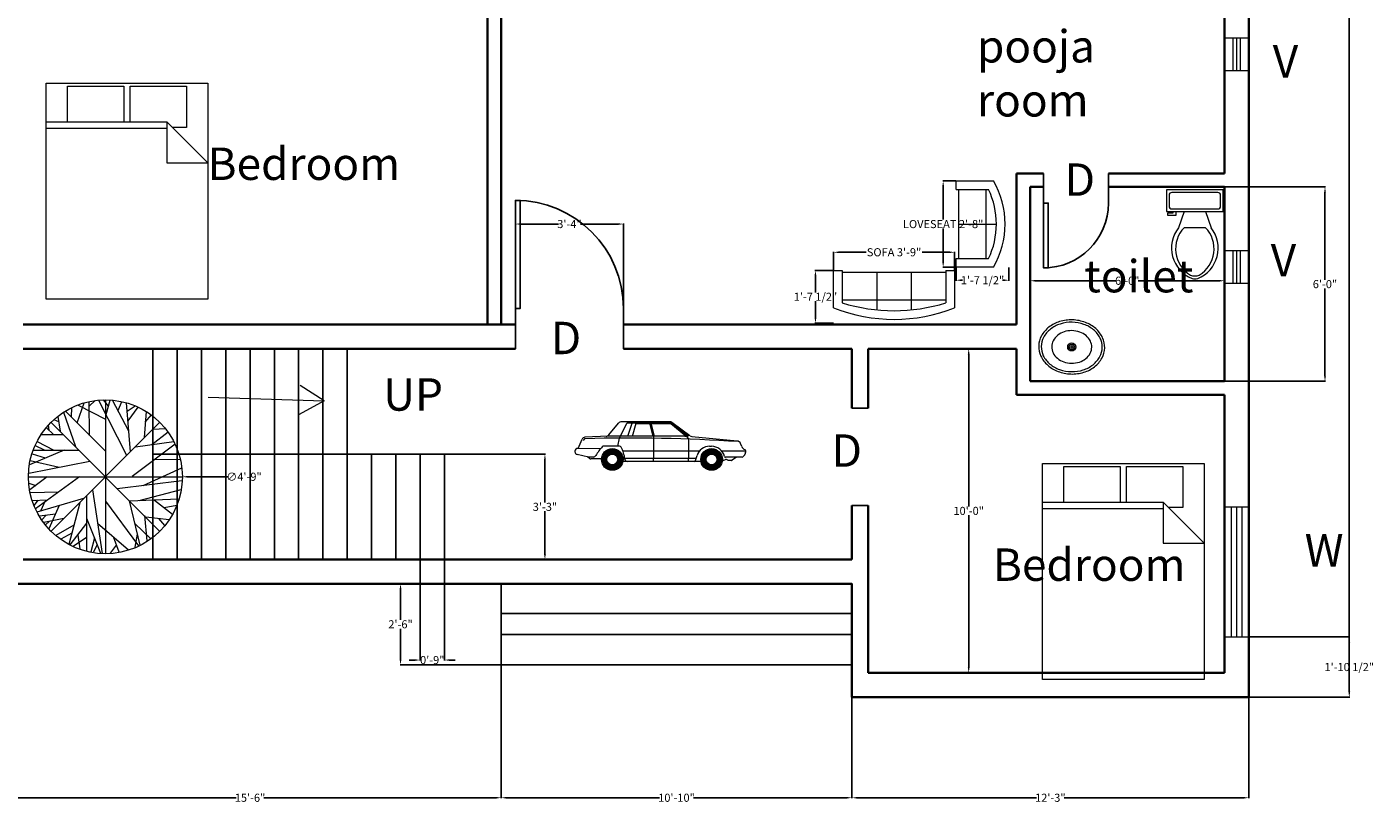
# Model space of a CAD drawing. Units: inches. Extents: x 751 to 1500, y 610 to 1297.
# Tile 2 of 4: x 1001 to 1500, y 610 to 898. Entities that reach past the tile are written whole.
import ezdxf

# ---------------------------------------------------------------- set-up
doc = ezdxf.new("R2010")
doc.units = ezdxf.units.IN
doc.header["$MEASUREMENT"] = 0
doc.layers.get('0').update_dxf_attribs({"color": 1})
for name, color, linetype, lineweight in [('A-ANNO-DIMS', 5, 'Continuous', 18), ('A-ANNO-SYMB', 7, 'Continuous', 18), ('A-ANNO-TEXT', 7, 'Continuous', 18), ('A-AREA-IDEN', 7, 'Continuous', 25), ('A-FLOR-FIXT', 9, 'Continuous', 18), ('A-FURN', 8, 'Continuous', 18), ('A-SITE-VEHI', 8, 'Continuous', 13), ('door', 2, 'Continuous', 25), ('L-PLNT', 3, 'Continuous', 13), ('stair', 130, 'Continuous', 25), ('wall', 6, 'Continuous', 35), ('windows', 70, 'Continuous', 18)]:
    doc.layers.add(name, color=color, linetype=linetype, lineweight=lineweight)
doc.styles.get("Standard").update_dxf_attribs({"font": 'arial.ttf'})
doc.dimstyles.get("Standard").update_dxf_attribs({"dimtxt": 3, "dimasz": 2, "dimexe": 0.18, "dimexo": 0.0625, "dimgap": 0.09, "dimtad": 0, "dimtih": 1, "dimtoh": 1, "dimdec": 0, "dimzin": 0, "dimdsep": 46, "dimlunit": 3, "dimtxsty": 'Standard', "dimcen": 0.09, "dimadec": 0, "dimazin": 0, "dimtfac": 1, "dimtdec": 0, "dimtofl": 0, "dimtmove": 0, "dimatfit": 3, "dimfxl": 1, "dimtolj": 1, "dimtzin": 0, "dimarcsym": 0})

# ---------------------------------------------------------------- blocks, each defined once
blk = doc.blocks.new('*U5')
for p, q in [((-24, 0), (-24, 6)), ((0, 0), (0, 6))]:
    blk.add_line(p, q)
blk.add_lwpolyline([(0, 0), (0, -24), (-1.75, -24), (-1.75, 0)], close=True)
blk.add_arc((0, 0), 24, 180, 270)
blk = doc.blocks.new('*U6')
for p, q in [((-40, 0), (-40, -6)), ((0, 0), (0, -6))]:
    blk.add_line(p, q)
blk.add_lwpolyline([(0, 0), (0, 40), (-1.75, 40), (-1.75, 0)], close=True)
blk.add_arc((0, 0), 40, 90, 180)
blk = doc.blocks.new('Car - sedan  side')
for p, q in [((-139.5, 36), (-129.6, 47.9)), ((-128.6, 32.6), (-121.2, 48)), ((-77.8, 49.3), (-126.6, 49.3)), ((-74.7, 48), (-121.2, 48)), ((-120.3, 34.7), (-115.7, 48)), ((-115.4, 34.7), (-111.7, 48)), ((-97.5, 47.3), (-111.9, 47.3)), ((-94.4, 34.7), (-97.7, 48)), ((-93.7, 34.7), (-97, 48)), ((-93, 34.7), (-96.3, 48)), ((-76.3, 47.3), (-96.2, 47.3)), ((-61.1, 34.7), (-76.3, 47.3)), ((-60, 34.6), (-76.1, 48)), ((-56.9, 35.1), (-75.5, 48.6)), ((-58.5, 34.9), (-75, 48)), ((-170.9, 22.3), (-166.8, 31.6)), ((-164.6, 31.6), (-165.5, 30.4)), ((-140.2, 34.7), (-163.9, 33.6)), ((-62.3, 34.7), (-140.2, 34.7)), ((-130.4, 24.6), (-128.6, 32.6)), ((-93.7, 19.6), (-93.7, 34.7)), ((-62.3, 34.7), (-60, 34.6)), ((-60, 34.6), (-58.5, 34.9)), ((-58, 31.6), (-60, 34.6)), ((-57.2, 35.4), (-58.5, 34.9)), ((-58, 19.6), (-58, 31.6)), ((-54.9, 34.4), (-8.8, 29.8)), ((-174, 19.5), (-174, 18.9)), ((-160.1, 13.5), (-171.8, 16.2)), ((-148.3, 21.7), (-171.1, 22.3)), ((-128.8, 24.6), (-144.8, 24.6)), ((-47.2, 19.6), (-125.2, 19.6)), ((-93.7, 12.1), (-93.7, 19.6)), ((-58, 12.1), (-58, 19.6)), ((-51.4, 9.9), (-49.7, 15.1)), ((-37, 24.4), (-34.9, 24.4)), ((0, 19.6), (-24.7, 19.6)), ((-4.2, 24.2), (-5.4, 27.3)), ((-3.2, 13.6), (-1.8, 15)), ((-159.2, 12.1), (-161.1, 13.7)), ((-155, 13.5), (-160.1, 13.5)), ((-147, 11.6), (-157.7, 11.6)), ((-120.6, 9), (-125.2, 9)), ((-50.7, 12.1), (-123.3, 12.1)), ((-45.8, 9), (-120.6, 9)), ((-94.2, 9), (-94.2, 12.1)), ((-58.4, 9), (-58.4, 12.1)), ((-20.4, 11.1), (-24.1, 9.4)), ((-4.2, 13.2), (-20.7, 13.2)), ((-18.8, 10.4), (-19.1, 10.8)), ((-14.7, 10), (-18, 10)), ((-9.5, 13.2), (-14.1, 10.2))]:
    blk.add_line(p, q)
at = {"const_width": 5.49}
for points in [[(-127.8, 11, -1), (-144.3, 11, -1)], [(-26.7, 11, -1), (-43.2, 11, -1)]]:
    blk.add_lwpolyline(points, format="xyb", close=True, dxfattribs=at)
for centre, radius in [((-136, 11), 11), ((-136, 11), 5.51), ((-34.9, 11), 11), ((-34.9, 11), 5.51)]:
    blk.add_circle(centre, radius)
for centre, radius, start, end in [((-126.6, 45.4), 3.97, 90, 140.3029), ((-77.8, 45.4), 3.97, 54.135, 90), ((-163.7, 30.2), 3.38, 92.6827, 155.9736), ((-163.6, 30.9), 1.17, 91.491, 143.9553), ((-118.5, -1702.1), 1734.8, 86.347, 91.491), ((-142.6, 38.5), 3.97, 272.6827, 320.3029), ((-54.5, 38.3), 3.97, 234.135, 264.3123), ((-9.1, 25.8), 4, 21.3107, 84.3123), ((-171.2, 19.5), 2.82, 88.4193, 180), ((-171.2, 18.9), 2.82, 180, 257.0905), ((-155, 16.1), 2.62, 270, 332.9097), ((-118.1, -2.8), 38.8, 136.3964, 152.9097), ((-144.8, 22.6), 1.98, 90, 136.3964), ((-128.8, 22.6), 1.98, 28.1371, 90), ((-157.1, 7.5), 34.1, 6.5135, 28.1371), ((-37, 11), 13.4, 90, 161.9732), ((-34.9, 11), 13.4, 13.5864, 90), ((-20.7, 14.4), 1.24, 193.5864, 270), ((0.9, 26.2), 5.49, 201.3107, 247.7048), ((-3.8, 17.1), 2.96, 313.7173, 352.3839), ((-1.9, 19.3), 1.94, 325.3744, 67.7048), ((2.5, 16.3), 3.37, 145.3744, 172.3839), ((-157.7, 13.9), 2.32, 230.1291, 270), ((-120.6, 11.6), 2.62, 186.5135, 270), ((-52.6, 10.3), 1.24, 270, 341.9732), ((-19.9, 10.1), 1.06, 39.301, 113.7159), ((-18, 11.1), 1.06, 219.301, 270), ((-14.7, 11.1), 1.06, 270, 303.047), ((-4.2, 14.6), 1.46, 270, 313.7173)]:
    blk.add_arc(centre, radius, start, end)
blk = doc.blocks.new('Sofa - Roundback 7 ft.')
for p, q in [((-12.00002, -32.4421), (-12.00003, -6.5971)), ((11.99997, -32.4421), (11.99998, -6.5971)), ((-36.000027, -34), (-36.000027, -11.4696)), ((-35.999844, -13.3819), (35.9998, -13.3819)), ((35.99998, -34), (35.99998, -11.4696)), ((-36.000027, -32.4421), (35.99998, -32.4421))]:
    blk.add_line(p, q)
for points in [[(-36.000027, -34), (-42.000027, -34), (-42.000027, -8)], [(41.99998, -8), (41.99998, -34), (35.99998, -34)]]:
    blk.add_lwpolyline(points)
for centre, radius, start, end in [((0, -114.25), 114.25, 68.43141, 111.5686), ((-0.00001, -127.1968), 121.1968, 72.72033, 107.2797)]:
    blk.add_arc(centre, radius, start, end)
blk = doc.blocks.new('Sofa - Roundback Loveseat 5 ft.')
for p, q in [((0, -32.44198), (0, -5.99998)), ((-24, -33.99998), (-24, -11.46958)), ((-23.9998, -13.38178), (23.99986, -13.38178)), ((24.00004, -33.99998), (24.00004, -11.46958)), ((-24, -32.44198), (24.00004, -32.44198))]:
    blk.add_line(p, q)
for points in [[(-24, -33.99998), (-30, -33.99998), (-30, -7.99998)], [(30.00004, -7.99998), (30.00004, -33.99998), (24.00004, -33.99998)]]:
    blk.add_lwpolyline(points)
for centre, radius, start, end in [((0, -60.24998), 60.24998, 60.13715, 119.8628), ((0, -61.38438), 55.38444, 64.32083, 115.6792)]:
    blk.add_arc(centre, radius, start, end)
blk = doc.blocks.new('Bed - Queen')
for p, q in [((0, -80.00003), (0, 0)), ((0, 0), (59.99999, 0)), ((59.99999, 0), (59.99999, -80.00003)), ((7.99999, -1.2), (28.79998, -1.2)), ((7.99999, -14.4), (7.99999, -1.2)), ((28.79998, -1.2), (28.79998, -14.4)), ((31.19999, -1.2), (51.99999, -1.2)), ((31.19999, -14.4), (31.19999, -1.2)), ((51.99999, -1.2), (51.99999, -16.4)), ((0, -14.4), (44.8, -14.4)), ((59.99999, -29.6), (44.8, -14.4)), ((44.8, -14.4), (44.8, -29.6)), ((44.8, -16.8), (0, -16.8)), ((51.99999, -16.4), (46.79936, -16.4)), ((44.8, -29.6), (59.99999, -29.6)), ((59.99999, -80.00003), (0, -80.00003))]:
    blk.add_line(p, q)
blk = doc.blocks.new('Tree - deciduous plan')
for p, q in [((-26.4472, 46.5894), (-26.2712, 53.8116)), ((-22.0458, 42.0753), (-16.5881, 57.6486)), ((-21.1656, 55.8436), (-0.0388, 45.0094)), ((-12.5388, 54.9406), (-7.9613, 59.4546)), ((-12.3627, 32.1443), (-12.5388, 58.7776)), ((-5.3205, 59.6806), (16.5105, 16.7963)), ((2.426, 54.9406), (-1.4472, 59.9056)), ((0, 59.9996), (0, -60)), ((0.4894, 48.6208), (3.6584, 59.6806)), ((18.2711, 35.5298), (5.419, 59.6806)), ((9.8203, 51.5549), (12.8133, 58.5516)), ((19.6795, 19.5047), (16.3344, 57.6486)), ((17.0387, 51.1035), (23.2006, 55.1666)), ((17.7429, 43.6552), (25.4894, 54.2636)), ((42, 42), (-42, -42)), ((42, -42), (-42, 42)), ((-40.1797, 44.558), (-36.4825, 43.2038)), ((-37.0107, 47.0408), (-35.25, 35.5298)), ((-32.6092, 50.4264), (-23.2782, 23.5674)), ((-31.2008, 51.1035), (-0.2149, 20.1818)), ((31.6513, 50.8778), (30.2429, 30.5643)), ((31.1232, 42.5267), (35.8767, 48.1693)), ((-49.8627, 32.8214), (-32.7853, 32.8214)), ((-45.8134, 38.2383), (-40.5318, 33.0471)), ((-43.8768, 36.4326), (-44.405, 40.2696)), ((36.2288, 25.1474), (48.9049, 35.0784)), ((37.1091, 37.1098), (46.6161, 37.5612)), ((-54.7923, 24.4702), (-47.75, 21.0847)), ((-53.2078, 27.4044), (-40.1797, 20.859)), ((54.3626, 25.3731), (20.9119, 0.3198)), ((23.3767, 23.3417), (53.3063, 27.4044)), ((-59.7219, 2.8025), (-12.0106, 12.0565)), ((-32.2571, 20.6333), (-59.1937, 9.348)), ((-58.6656, 12.7336), (-35.9543, 7.5424)), ((-57.081, 17.9248), (-47.0458, 14.7649)), ((-56.0247, 20.859), (-20.8134, 20.859)), ((38.5175, 13.4107), (58.2359, 13.6364)), ((-54.6162, -24.7335), (-20.2853, 0.0941)), ((29.3626, -6.6771), (59.4682, 7.091)), ((-60, 0), (60, 0)), ((-59.7219, -4.8714), (-54.2641, -6.6771)), ((-45.2853, -0.1316), (-59.0177, -10.0627)), ((-10.074, -10.0627), (-2.5036, -59.7178)), ((9.2922, -9.1598), (59.6443, -2.8401)), ((26.3697, -18.4138), (58.9401, -9.8369)), ((-58.4895, -12.3197), (-36.4825, -11.6426)), ((-57.081, -18.4138), (-45.2853, -17.9624)), ((-52.6797, -18.188), (-55.4966, -22.0251)), ((-53.2078, -27.442), (-16.7641, -16.6081)), ((-47.2219, -19.3166), (-50.2148, -26.3135)), ((-19.9331, -20.2194), (-28.5599, -52.721)), ((-14.8275, -15.0282), (-14.6515, -57.6865)), ((-0.0388, -19.0909), (25.8415, -53.8495)), ((18.6232, -18.6394), (26.7218, -53.3981)), ((18.7992, -18.6394), (57.3556, -17.2853)), ((38.1654, -18.188), (52.426, -29.0219)), ((-38.9472, -29.0219), (-51.4472, -30.6018)), ((-46.5177, -30.1504), (-49.5106, -33.536)), ((-35.9543, -22.4765), (-44.0529, -40.5329)), ((30.419, -30.1504), (32.3556, -50.0125)), ((31.4753, -31.279), (49.6091, -33.3103)), ((45.9119, -24.0564), (55.595, -22.2508)), ((-32.4331, -32.4075), (-48.1021, -35.5674)), ((-43.7008, -34.6645), (-46.6937, -37.373)), ((-24.6867, -37.8244), (-38.7712, -45.7241)), ((-14.6515, -36.2445), (-27.6797, -52.9467)), ((-14.6515, -32.1818), (-3.912, -59.4922)), ((-6.2008, -36.2445), (17.919, -57.0094)), ((22.8485, -36.4702), (35.3485, -48.4326)), ((41.5105, -32.6332), (46.088, -38.0501)), ((-26.2712, -43.9185), (-34.7219, -48.6583)), ((-14.6515, -47.3041), (-25.0388, -54.3009)), ((-21.5177, -45.4984), (-19.9331, -56.1065)), ((-8.4895, -47.5298), (-11.4825, -58.5893)), ((5.9471, -46.6269), (10.5246, -58.5893)), ((24.7852, -44.8213), (23.0246, -54.978)), ((-6.3768, -52.721), (-9.3698, -58.815)), ((8.4119, -53.1724), (3.8344, -59.4922))]:
    blk.add_line(p, q)
blk.add_circle((0, 0), 60)
blk = doc.blocks.new('Sink - Oval top')
for p, q in [((-1, 0), (1, 0)), ((0, 1), (0, -1))]:
    blk.add_line(p, q)
for points in [[(-12.23, 0.39, 0.117634), (-11.46, -3.36, 0.104469), (-8.88, -6.8, 0.090016), (-5.08, -9.07, 0.08192), (-0.32, -10.02, 0.08192), (4.49, -9.38, 0.090016), (8.42, -7.36, 0.104469), (11.22, -4.09, 0.117634), (12.23, -0.39, 0.117634), (11.46, 3.36, 0.104469), (8.88, 6.8, 0.090016), (5.08, 9.07, 0.08192), (0.32, 10.02, 0.08192), (-4.49, 9.38, 0.090016), (-8.42, 7.36, 0.104469), (-11.22, 4.09, 0.117634)], [(-11.29, 0.16, 0.118622), (-10.52, -3.25, 0.104678), (-8.07, -6.36, 0.089562), (-4.54, -8.37, 0.081185), (-0.13, -9.15, 0.081185), (4.3, -8.49, 0.089562), (7.89, -6.58, 0.104678), (10.42, -3.55, 0.118622), (11.29, -0.16, 0.118622), (10.52, 3.25, 0.104678), (8.07, 6.36, 0.089562), (4.54, 8.37, 0.081185), (0.13, 9.15, 0.081185), (-4.3, 8.49, 0.089562), (-7.89, 6.58, 0.104678), (-10.42, 3.55, 0.118622)], [(-7.42, 0.08, 0.118283), (-6.91, -2.17, 0.104607), (-5.29, -4.21, 0.089718), (-2.97, -5.53, 0.081436), (-0.07, -6.04, 0.081436), (2.84, -5.59, 0.089718), (5.2, -4.33, 0.104607), (6.86, -2.32, 0.118283), (7.42, -0.08, 0.118283), (6.91, 2.17, 0.104607), (5.29, 4.21, 0.089718), (2.97, 5.53, 0.081436), (0.07, 6.04, 0.081436), (-2.84, 5.59, 0.089718), (-5.2, 4.33, 0.104607), (-6.86, 2.32, 0.118283)]]:
    blk.add_lwpolyline(points, format="xyb", close=True)
for radius in [1.5, 1]:
    blk.add_circle((0, 0), radius)
blk = doc.blocks.new('Toilet - top')
for p, q in [((9.5, -6), (9.5, -2)), ((-10, -8.5), (-8, -8.5)), ((-10, -9.5), (-10, -8.5)), ((-7, -9.5), (-10, -9.5)), ((-8, -8.5), (-8, -8)), ((-7, -8), (-7, -9.5)), ((-4, -8), (-6, -14)), ((4, -8), (6, -14)), ((4, -14), (-4, -14))]:
    blk.add_line(p, q)
blk.add_lwpolyline([(10.5, -8), (10.5, 0), (-10.5, 0), (-10.5, -8)], close=True)
for points in [[(-9.5, -2), (-9.5, -6)], [(8.5, -1), (-8.5, -1)], [(-8.5, -7), (8.5, -7)]]:
    blk.add_lwpolyline(points)
for centre, radius, start, end in [((-8.62, -1.88), 0.884, 81.8699, 188.1301), ((8.62, -1.88), 0.884, 351.8699, 98.1301), ((-8.62, -6.12), 0.884, 171.8699, 278.1301), ((8.62, -6.12), 0.884, 261.8699, 8.1301), ((3.52, -21.58), 12.17, 141.4691, 247.9714), ((4.2, -21.82), 11.33, 136.3677, 238.9468), ((-3.52, -21.58), 12.17, 292.0284, 38.5307), ((-4.2, -21.82), 11.33, 301.053, 43.6321), ((0, -27.88), 4, 245.7318, 294.2682), ((0, -29), 4, 254.8605, 285.1395)]:
    blk.add_arc(centre, radius, start, end)
blk = doc.blocks.new('WIN-48IN-PLAN')
for p, q in [((2.5, 48), (2.5, 0)), ((4.5, 48), (4.5, 0)), ((6.5, 48), (6.5, 0))]:
    blk.add_line(p, q)
blk.add_lwpolyline([(9, 48), (0, 48), (0, 0), (9, 0)], close=True)
blk = doc.blocks.new('VENT-12IN-PLAN')
for p, q in [((3.14, 12), (3.14, 0)), ((4.5, 12), (4.5, 0)), ((5.86, 12), (5.86, 0))]:
    blk.add_line(p, q)
blk.add_lwpolyline([(0, 0), (9, 0), (9, 12), (0, 12)], close=True)
blk = doc.blocks.new('*D41')
at = {"layer": 'A-ANNO-DIMS', "color": 0, "lineweight": -2, "transparency": 16777216}
for p, q in [((1300.18, 807.83), (1300.18, 814.67)), ((1302.18, 814.49), (1312.21, 814.49)), ((1342.97, 814.49), (1332.93, 814.49)), ((1344.97, 807.83), (1344.97, 814.67))]:
    blk.add_line(p, q, dxfattribs=at)
at = {"layer": 'A-ANNO-DIMS', "color": 0, "transparency": 16777216}
for points in [[(1302.18, 814.82), (1302.18, 814.16), (1300.18, 814.49)], [(1342.97, 814.82), (1342.97, 814.16), (1344.97, 814.49)]]:
    blk.add_solid(points, dxfattribs=at)
at = {"layer": 'Defpoints', "color": 0, "transparency": 16777216}
for p in [(1300.18, 814.49), (1300.18, 807.77), (1344.97, 807.77)]:
    blk.add_point(p, dxfattribs=at)
at = {"layer": 'A-ANNO-DIMS', "color": 0, "transparency": 16777216, "insert": (1322.57, 814.49), "char_height": 3, "attachment_point": 5}
blk.add_mtext('\\A1;SOFA 3\'-9"', dxfattribs=at)
blk = doc.blocks.new('*D42')
at = {"layer": 'A-ANNO-DIMS', "color": 0, "lineweight": -2, "transparency": 16777216}
for p, q in [((1300.11, 807.77), (1293.28, 807.77)), ((1293.46, 805.77), (1293.46, 799.64)), ((1293.46, 790.22), (1293.46, 796.36)), ((1300.11, 788.22), (1293.28, 788.22))]:
    blk.add_line(p, q, dxfattribs=at)
at = {"layer": 'A-ANNO-DIMS', "color": 0, "transparency": 16777216}
for points in [[(1293.12, 805.77), (1293.79, 805.77), (1293.46, 807.77)], [(1293.12, 790.22), (1293.79, 790.22), (1293.46, 788.22)]]:
    blk.add_solid(points, dxfattribs=at)
at = {"layer": 'Defpoints', "color": 0, "transparency": 16777216}
for p in [(1300.18, 807.77), (1293.46, 788.22), (1300.18, 788.22)]:
    blk.add_point(p, dxfattribs=at)
at = {"layer": 'A-ANNO-DIMS', "color": 0, "transparency": 16777216, "insert": (1293.46, 798), "char_height": 3, "attachment_point": 5}
blk.add_mtext('\\A1;1\'-7 1/2"', dxfattribs=at)
blk = doc.blocks.new('*D43')
at = {"layer": 'A-ANNO-DIMS', "color": 0, "lineweight": -2, "transparency": 16777216}
for p, q in [((1345.51, 840.93), (1340.59, 840.93)), ((1340.77, 838.93), (1340.77, 826.57)), ((1340.77, 810.93), (1340.77, 823.29)), ((1345.51, 808.93), (1340.59, 808.93))]:
    blk.add_line(p, q, dxfattribs=at)
at = {"layer": 'A-ANNO-DIMS', "color": 0, "transparency": 16777216}
for points in [[(1340.44, 838.93), (1341.1, 838.93), (1340.77, 840.93)], [(1340.44, 810.93), (1341.1, 810.93), (1340.77, 808.93)]]:
    blk.add_solid(points, dxfattribs=at)
at = {"layer": 'Defpoints', "color": 0, "transparency": 16777216}
for p in [(1345.57, 840.93), (1340.77, 808.93), (1345.57, 808.93)]:
    blk.add_point(p, dxfattribs=at)
at = {"layer": 'A-ANNO-DIMS', "color": 0, "transparency": 16777216, "insert": (1340.77, 824.93), "char_height": 3, "attachment_point": 5}
blk.add_mtext('\\A1;LOVESEAT 2\'-8"', dxfattribs=at)
blk = doc.blocks.new('*D44')
at = {"layer": 'A-ANNO-DIMS', "color": 0, "lineweight": -2, "transparency": 16777216}
for p, q in [((1345.57, 808.87), (1345.57, 803.95)), ((1365.12, 808.87), (1365.12, 803.95)), ((1347.57, 804.13), (1347.91, 804.13)), ((1363.12, 804.13), (1362.78, 804.13))]:
    blk.add_line(p, q, dxfattribs=at)
at = {"layer": 'A-ANNO-DIMS', "color": 0, "transparency": 16777216}
for points in [[(1347.57, 804.47), (1347.57, 803.8), (1345.57, 804.13)], [(1363.12, 804.47), (1363.12, 803.8), (1365.12, 804.13)]]:
    blk.add_solid(points, dxfattribs=at)
at = {"layer": 'Defpoints', "color": 0, "transparency": 16777216}
for p in [(1345.57, 808.93), (1365.12, 808.93), (1365.12, 804.13)]:
    blk.add_point(p, dxfattribs=at)
at = {"layer": 'A-ANNO-DIMS', "color": 0, "transparency": 16777216, "insert": (1355.34, 804.13), "char_height": 3, "attachment_point": 5}
blk.add_mtext('\\A1;1\'-7 1/2"', dxfattribs=at)
blk = doc.blocks.new('*D45')
at = {"layer": 'A-ANNO-DIMS', "color": 0, "lineweight": -2, "transparency": 16777216}
for p, q in [((1454.04, 1205.69), (1491.41, 1205.69)), ((1491.23, 1203.69), (1491.23, 929.31)), ((1491.23, 651.69), (1491.23, 926.07)), ((1454.04, 649.69), (1491.41, 649.69))]:
    blk.add_line(p, q, dxfattribs=at)
at = {"layer": 'A-ANNO-DIMS', "color": 0, "transparency": 16777216}
for points in [[(1490.9, 1203.69), (1491.57, 1203.69), (1491.23, 1205.69)], [(1490.9, 651.69), (1491.57, 651.69), (1491.23, 649.69)]]:
    blk.add_solid(points, dxfattribs=at)
at = {"layer": 'Defpoints', "color": 0, "transparency": 16777216}
for p in [(1453.98, 1205.69), (1491.23, 1205.69), (1453.98, 649.69)]:
    blk.add_point(p, dxfattribs=at)
at = {"layer": 'A-ANNO-DIMS', "color": 0, "transparency": 16777216, "insert": (1491.23, 927.69), "char_height": 3, "attachment_point": 5}
blk.add_mtext('\\A1;46\'-4"', dxfattribs=at)
blk = doc.blocks.new('*D46')
at = {"layer": 'A-ANNO-DIMS', "color": 0, "lineweight": -2, "transparency": 16777216}
for p, q in [((1306.98, 649.63), (1306.98, 612.26)), ((1453.98, 649.63), (1453.98, 612.26)), ((1308.98, 612.44), (1375.38, 612.44)), ((1451.98, 612.44), (1385.58, 612.44))]:
    blk.add_line(p, q, dxfattribs=at)
at = {"layer": 'A-ANNO-DIMS', "color": 0, "transparency": 16777216}
for points in [[(1308.98, 612.77), (1308.98, 612.11), (1306.98, 612.44)], [(1451.98, 612.77), (1451.98, 612.11), (1453.98, 612.44)]]:
    blk.add_solid(points, dxfattribs=at)
at = {"layer": 'Defpoints', "color": 0, "transparency": 16777216}
for p in [(1306.98, 649.69), (1453.98, 649.69), (1453.98, 612.44)]:
    blk.add_point(p, dxfattribs=at)
at = {"layer": 'A-ANNO-DIMS', "color": 0, "transparency": 16777216, "insert": (1380.48, 612.44), "char_height": 3, "attachment_point": 5}
blk.add_mtext('\\A1;12\'-3"', dxfattribs=at)
blk = doc.blocks.new('*D47')
at = {"layer": 'A-ANNO-DIMS', "color": 0, "lineweight": -2, "transparency": 16777216}
for p, q in [((990.98, 691.63), (990.98, 612.26)), ((1176.98, 691.63), (1176.98, 612.26)), ((992.98, 612.44), (1078.88, 612.44)), ((1174.98, 612.44), (1089.08, 612.44))]:
    blk.add_line(p, q, dxfattribs=at)
at = {"layer": 'A-ANNO-DIMS', "color": 0, "transparency": 16777216}
for points in [[(992.98, 612.77), (992.98, 612.11), (990.98, 612.44)], [(1174.98, 612.77), (1174.98, 612.11), (1176.98, 612.44)]]:
    blk.add_solid(points, dxfattribs=at)
at = {"layer": 'Defpoints', "color": 0, "transparency": 16777216}
for p in [(990.98, 691.69), (1176.98, 691.69), (1176.98, 612.44)]:
    blk.add_point(p, dxfattribs=at)
at = {"layer": 'A-ANNO-DIMS', "color": 0, "transparency": 16777216, "insert": (1083.98, 612.44), "char_height": 3, "attachment_point": 5}
blk.add_mtext('\\A1;15\'-6"', dxfattribs=at)
blk = doc.blocks.new('*D48')
at = {"layer": 'A-ANNO-DIMS', "color": 0, "lineweight": -2, "transparency": 16777216}
for p, q in [((1176.98, 661.63), (1176.98, 612.26)), ((1306.98, 661.63), (1306.98, 612.26)), ((1178.98, 612.44), (1235.72, 612.44)), ((1304.98, 612.44), (1248.25, 612.44))]:
    blk.add_line(p, q, dxfattribs=at)
at = {"layer": 'A-ANNO-DIMS', "color": 0, "transparency": 16777216}
for points in [[(1178.98, 612.77), (1178.98, 612.11), (1176.98, 612.44)], [(1304.98, 612.77), (1304.98, 612.11), (1306.98, 612.44)]]:
    blk.add_solid(points, dxfattribs=at)
at = {"layer": 'Defpoints', "color": 0, "transparency": 16777216}
for p in [(1176.98, 661.69), (1306.98, 661.69), (1306.98, 612.44)]:
    blk.add_point(p, dxfattribs=at)
at = {"layer": 'A-ANNO-DIMS', "color": 0, "transparency": 16777216, "insert": (1241.98, 612.44), "char_height": 3, "attachment_point": 5}
blk.add_mtext('\\A1;10\'-10"', dxfattribs=at)
blk = doc.blocks.new('*D52')
at = {"layer": 'A-ANNO-DIMS', "color": 0, "lineweight": -2, "transparency": 16777216}
for p, q in [((1445.04, 838.69), (1482.41, 838.69)), ((1482.23, 836.69), (1482.23, 804.31)), ((1482.23, 768.69), (1482.23, 801.07)), ((1445.04, 766.69), (1482.41, 766.69))]:
    blk.add_line(p, q, dxfattribs=at)
at = {"layer": 'A-ANNO-DIMS', "color": 0, "transparency": 16777216}
for points in [[(1481.9, 836.69), (1482.57, 836.69), (1482.23, 838.69)], [(1481.9, 768.69), (1482.57, 768.69), (1482.23, 766.69)]]:
    blk.add_solid(points, dxfattribs=at)
at = {"layer": 'Defpoints', "color": 0, "transparency": 16777216}
for p in [(1444.98, 838.69), (1444.98, 766.69), (1482.23, 766.69)]:
    blk.add_point(p, dxfattribs=at)
at = {"layer": 'A-ANNO-DIMS', "color": 0, "transparency": 16777216, "insert": (1482.23, 802.69), "char_height": 3, "attachment_point": 5}
blk.add_mtext('\\A1;6\'-0"', dxfattribs=at)
blk = doc.blocks.new('*D53')
at = {"layer": 'A-ANNO-DIMS', "color": 0, "lineweight": -2, "transparency": 16777216}
for p, q in [((1313.04, 778.69), (1350.41, 778.69)), ((1350.23, 776.69), (1350.23, 720.31)), ((1350.23, 660.69), (1350.23, 717.07)), ((1313.04, 658.69), (1350.41, 658.69))]:
    blk.add_line(p, q, dxfattribs=at)
at = {"layer": 'A-ANNO-DIMS', "color": 0, "transparency": 16777216}
for points in [[(1349.9, 776.69), (1350.57, 776.69), (1350.23, 778.69)], [(1349.9, 660.69), (1350.57, 660.69), (1350.23, 658.69)]]:
    blk.add_solid(points, dxfattribs=at)
at = {"layer": 'Defpoints', "color": 0, "transparency": 16777216}
for p in [(1312.98, 778.69), (1312.98, 658.69), (1350.23, 658.69)]:
    blk.add_point(p, dxfattribs=at)
at = {"layer": 'A-ANNO-DIMS', "color": 0, "transparency": 16777216, "insert": (1350.23, 718.69), "char_height": 3, "attachment_point": 5}
blk.add_mtext('\\A1;10\'-0"', dxfattribs=at)
blk = doc.blocks.new('*D55')
at = {"layer": 'A-ANNO-DIMS', "color": 0, "lineweight": -2, "transparency": 16777216}
for p, q in [((1372.98, 766.75), (1372.98, 804.12)), ((1374.98, 803.94), (1404.9, 803.94)), ((1442.98, 803.94), (1413.07, 803.94)), ((1444.98, 766.75), (1444.98, 804.12))]:
    blk.add_line(p, q, dxfattribs=at)
at = {"layer": 'A-ANNO-DIMS', "color": 0, "transparency": 16777216}
for points in [[(1374.98, 804.27), (1374.98, 803.61), (1372.98, 803.94)], [(1442.98, 804.27), (1442.98, 803.61), (1444.98, 803.94)]]:
    blk.add_solid(points, dxfattribs=at)
at = {"layer": 'Defpoints', "color": 0, "transparency": 16777216}
for p in [(1444.98, 803.94), (1372.98, 766.69), (1444.98, 766.69)]:
    blk.add_point(p, dxfattribs=at)
at = {"layer": 'A-ANNO-DIMS', "color": 0, "transparency": 16777216, "insert": (1408.98, 803.94), "char_height": 3, "attachment_point": 5}
blk.add_mtext('\\A1;6\'-0"', dxfattribs=at)
blk = doc.blocks.new('*D57')
at = {"layer": 'A-ANNO-DIMS', "color": 0, "lineweight": -2, "transparency": 16777216}
for p, q in [((1182.32, 787.75), (1182.32, 825.12)), ((1184.32, 824.94), (1198.24, 824.94)), ((1220.32, 824.94), (1206.39, 824.94)), ((1222.32, 787.75), (1222.32, 825.12))]:
    blk.add_line(p, q, dxfattribs=at)
at = {"layer": 'A-ANNO-DIMS', "color": 0, "transparency": 16777216}
for points in [[(1184.32, 825.27), (1184.32, 824.61), (1182.32, 824.94)], [(1220.32, 825.27), (1220.32, 824.61), (1222.32, 824.94)]]:
    blk.add_solid(points, dxfattribs=at)
at = {"layer": 'Defpoints', "color": 0, "transparency": 16777216}
for p in [(1222.32, 824.94), (1182.32, 787.69), (1222.32, 787.69)]:
    blk.add_point(p, dxfattribs=at)
at = {"layer": 'A-ANNO-DIMS', "color": 0, "transparency": 16777216, "insert": (1202.32, 824.94), "char_height": 3, "attachment_point": 5}
blk.add_mtext('\\A1;3\'-4"', dxfattribs=at)
blk = doc.blocks.new('*D60')
at = {"layer": 'A-ANNO-DIMS', "color": 0, "lineweight": -2, "transparency": 16777216}
for p, q in [((1156.04, 739.69), (1193.41, 739.69)), ((1193.23, 737.69), (1193.23, 721.81)), ((1193.23, 702.69), (1193.23, 718.57)), ((1156.04, 700.69), (1193.41, 700.69))]:
    blk.add_line(p, q, dxfattribs=at)
at = {"layer": 'A-ANNO-DIMS', "color": 0, "transparency": 16777216}
for points in [[(1192.9, 737.69), (1193.57, 737.69), (1193.23, 739.69)], [(1192.9, 702.69), (1193.57, 702.69), (1193.23, 700.69)]]:
    blk.add_solid(points, dxfattribs=at)
at = {"layer": 'Defpoints', "color": 0, "transparency": 16777216}
for p in [(1155.98, 739.69), (1155.98, 700.69), (1193.23, 700.69)]:
    blk.add_point(p, dxfattribs=at)
at = {"layer": 'A-ANNO-DIMS', "color": 0, "transparency": 16777216, "insert": (1193.23, 720.19), "char_height": 3, "attachment_point": 5}
blk.add_mtext('\\A1;3\'-3"', dxfattribs=at)
blk = doc.blocks.new('*D61')
at = {"layer": 'A-ANNO-DIMS', "color": 0, "lineweight": -2, "transparency": 16777216}
for p, q in [((1146.98, 700.63), (1146.98, 663.26)), ((1155.98, 700.63), (1155.98, 663.26)), ((1144.98, 663.44), (1142.98, 663.44)), ((1157.98, 663.44), (1159.98, 663.44))]:
    blk.add_line(p, q, dxfattribs=at)
at = {"layer": 'A-ANNO-DIMS', "color": 0, "transparency": 16777216}
for points in [[(1144.98, 663.77), (1144.98, 663.11), (1146.98, 663.44)], [(1157.98, 663.77), (1157.98, 663.11), (1155.98, 663.44)]]:
    blk.add_solid(points, dxfattribs=at)
at = {"layer": 'Defpoints', "color": 0, "transparency": 16777216}
for p in [(1146.98, 700.69), (1155.98, 700.69), (1146.98, 663.44)]:
    blk.add_point(p, dxfattribs=at)
at = {"layer": 'A-ANNO-DIMS', "color": 0, "transparency": 16777216, "insert": (1151.48, 663.44), "char_height": 3, "attachment_point": 5}
blk.add_mtext('\\A1;0\'-9"', dxfattribs=at)
blk = doc.blocks.new('*D65')
at = {"layer": 'A-ANNO-DIMS', "color": 0, "lineweight": -2, "transparency": 16777216}
for p, q in [((1454.04, 672.06), (1491.41, 672.06)), ((1491.23, 670.06), (1491.23, 662.52)), ((1491.23, 651.69), (1491.23, 659.23)), ((1454.04, 649.69), (1491.41, 649.69))]:
    blk.add_line(p, q, dxfattribs=at)
at = {"layer": 'A-ANNO-DIMS', "color": 0, "transparency": 16777216}
for points in [[(1490.9, 670.06), (1491.57, 670.06), (1491.23, 672.06)], [(1490.9, 651.69), (1491.57, 651.69), (1491.23, 649.69)]]:
    blk.add_solid(points, dxfattribs=at)
at = {"layer": 'Defpoints', "color": 0, "transparency": 16777216}
for p in [(1453.98, 672.06), (1453.98, 649.69), (1491.23, 649.69)]:
    blk.add_point(p, dxfattribs=at)
at = {"layer": 'A-ANNO-DIMS', "color": 0, "transparency": 16777216, "insert": (1491.23, 660.87), "char_height": 3, "attachment_point": 5}
blk.add_mtext('\\A1;1\'-10 1/2"', dxfattribs=at)
blk = doc.blocks.new('*D67')
at = {"layer": 'A-ANNO-DIMS', "color": 0, "lineweight": -2, "transparency": 16777216}
for p, q in [((1176.92, 691.69), (1139.55, 691.69)), ((1139.73, 689.69), (1139.73, 678.31)), ((1139.73, 663.69), (1139.73, 675.07)), ((1176.92, 661.69), (1139.55, 661.69))]:
    blk.add_line(p, q, dxfattribs=at)
at = {"layer": 'A-ANNO-DIMS', "color": 0, "transparency": 16777216}
for points in [[(1139.4, 689.69), (1140.07, 689.69), (1139.73, 691.69)], [(1139.4, 663.69), (1140.07, 663.69), (1139.73, 661.69)]]:
    blk.add_solid(points, dxfattribs=at)
at = {"layer": 'Defpoints', "color": 0, "transparency": 16777216}
for p in [(1139.73, 691.69), (1176.98, 691.69), (1176.98, 661.69)]:
    blk.add_point(p, dxfattribs=at)
at = {"layer": 'A-ANNO-DIMS', "color": 0, "transparency": 16777216, "insert": (1139.73, 676.69), "char_height": 3, "attachment_point": 5}
blk.add_mtext('\\A1;2\'-6"', dxfattribs=at)
blk = doc.blocks.new('*D68')
at = {"layer": 'A-ANNO-DIMS', "color": 0, "lineweight": -2, "transparency": 16777216}
for p, q in [((1030.3, 731.33), (1030.48, 731.33)), ((1030.39, 731.24), (1030.39, 731.42)), ((1076.02, 731.33), (1060.91, 731.33))]:
    blk.add_line(p, q, dxfattribs=at)
at = {"layer": 'A-ANNO-DIMS', "color": 0, "transparency": 16777216}
blk.add_solid([(1060.91, 731.66), (1060.91, 730.99), (1058.91, 731.33)], dxfattribs=at)
at = {"layer": 'Defpoints', "color": 0, "transparency": 16777216}
for p in [(1001.88, 731.33), (1058.91, 731.33)]:
    blk.add_point(p, dxfattribs=at)
at = {"layer": 'A-ANNO-DIMS', "color": 0, "transparency": 16777216, "insert": (1081.73, 731.33), "char_height": 3, "attachment_point": 5}
blk.add_mtext('\\A1;∅4\'-9"', dxfattribs=at)

msp = doc.modelspace()

# ---------------------------------------------------------------- linework, layer by layer
at = {"layer": 'A-ANNO-SYMB'}
for p, q in [((1111.4, 759.47), (1102.57, 765.17)), ((1068.43, 760.83), (1111.4, 759.47)), ((1111.4, 759.47), (1102.23, 754.34))]:
    msp.add_line(p, q, dxfattribs=at)
at = {"layer": 'door'}
for p, q in [((1377.98, 838.69), (1377.98, 843.69)), ((1401.98, 838.69), (1401.98, 843.69)), ((1182.32, 787.69), (1182.32, 778.69)), ((1222.32, 787.69), (1222.32, 778.69)), ((1312.98, 756.69), (1306.98, 756.69)), ((1312.98, 720.69), (1306.98, 720.69))]:
    msp.add_line(p, q, dxfattribs=at)
at = {"layer": 'stair'}
for p, q in [((1047.98, 700.69), (1047.98, 778.69)), ((1056.98, 700.69), (1056.98, 778.69)), ((1065.98, 700.69), (1065.98, 778.69)), ((1074.98, 700.69), (1074.98, 778.69)), ((1083.98, 700.69), (1083.98, 778.69)), ((1092.98, 700.69), (1092.98, 778.69)), ((1101.98, 700.69), (1101.98, 778.69)), ((1110.98, 700.69), (1110.98, 778.69)), ((1119.98, 700.69), (1119.98, 778.69)), ((1119.98, 700.69), (1119.98, 778.69)), ((1119.98, 700.69), (1119.98, 778.69)), ((1047.98, 739.69), (1155.98, 739.69)), ((1128.98, 700.69), (1128.98, 739.69)), ((1137.98, 700.69), (1137.98, 739.69)), ((1146.98, 700.69), (1146.98, 739.69)), ((1155.98, 700.69), (1155.98, 739.69)), ((1176.98, 677.94), (1176.98, 685.69)), ((1306.98, 685.69), (1306.98, 677.94)), ((1176.98, 680.65), (1306.98, 680.65)), ((1306.98, 672.9), (1176.98, 672.9))]:
    msp.add_line(p, q, dxfattribs=at)
msp.add_lwpolyline([(1176.98, 691.69), (1306.98, 691.69), (1306.98, 661.69), (1176.98, 661.69)], close=True, dxfattribs=at)
at = {"layer": 'wall'}
for p, q in [((1453.98, 952.69), (1453.98, 850.69)), ((1444.98, 915.69), (1444.98, 850.69)), ((1171.98, 787.69), (1171.98, 902.69)), ((1176.98, 787.69), (1176.98, 902.69)), ((1444.98, 850.69), (1444.98, 843.69)), ((1453.98, 850.69), (1453.98, 796.69)), ((1367.98, 843.69), (1377.98, 843.69)), ((1367.98, 843.69), (1367.98, 787.69)), ((1401.98, 843.69), (1444.98, 843.69)), ((1372.98, 838.69), (1372.98, 766.69)), ((1372.98, 838.69), (1377.98, 838.69)), ((1401.98, 838.69), (1444.98, 838.69)), ((1444.98, 838.69), (1444.98, 796.69)), ((1444.98, 796.69), (1444.98, 766.69)), ((1453.98, 796.69), (1453.98, 649.69)), ((1182.32, 787.69), (999.98, 787.69)), ((1367.98, 787.69), (1222.32, 787.69)), ((1182.32, 778.69), (999.98, 778.69)), ((1306.98, 778.69), (1222.32, 778.69)), ((1306.98, 778.69), (1306.98, 756.69)), ((1367.98, 778.69), (1312.98, 778.69)), ((1312.98, 778.69), (1312.98, 756.69)), ((1367.98, 778.69), (1367.98, 761.69)), ((1372.98, 766.69), (1377.98, 766.69)), ((1372.98, 766.69), (1444.98, 766.69)), ((1367.98, 761.69), (1444.98, 761.69)), ((1444.98, 761.69), (1444.98, 658.69)), ((1306.98, 720.69), (1306.98, 700.69)), ((1312.98, 720.69), (1312.98, 658.69)), ((1306.98, 700.69), (999.98, 700.69)), ((1171.98, 691.69), (990.98, 691.69)), ((1306.98, 691.69), (1171.98, 691.69)), ((1306.98, 649.69), (1306.98, 691.69)), ((1444.98, 658.69), (1312.98, 658.69)), ((1453.98, 649.69), (1306.98, 649.69))]:
    msp.add_line(p, q, dxfattribs=at)

# ---------------------------------------------------------------- block references
at = {"layer": 'A-FLOR-FIXT'}
for name, p in [('Toilet - top', (1434.02, 837.59)), ('Sink - Oval top', (1388.4, 779.42)), ('Sink - Oval top', (1388.4, 779.42))]:
    msp.add_blockref(name, p, dxfattribs=at)
at = {"layer": 'A-FURN'}
for p in [(1008.39, 877.16), (1377.53, 736.3), (1377.53, 736.3)]:
    msp.add_blockref('Bed - Queen', p, dxfattribs=at)
at = {"layer": 'A-FURN', "xscale": 0.5332194670571152, "yscale": 0.5332194670571152, "zscale": 0.5332194670571152}
for name, p, rotation in [('Sofa - Roundback Loveseat 5 ft.', (1363.7, 824.93), 270), ('Sofa - Roundback 7 ft.', (1322.57, 789.64), 180)]:
    msp.add_blockref(name, p, dxfattribs=dict(at, rotation=rotation))
at = {"layer": 'A-SITE-VEHI', "xscale": 0.3638935471290085, "yscale": 0.3638935471290085, "zscale": 0.3638935471290085}
msp.add_blockref('Car - sedan  side', (1267.68, 733.74), dxfattribs=at)
at = {"layer": 'door', "xscale": -1, "rotation": 359.9999999999973}
for name, p in [('*U5', (1377.98, 832.69)), ('*U6', (1182.32, 793.69))]:
    msp.add_blockref(name, p, dxfattribs=at)
at = {"layer": 'L-PLNT', "xscale": 0.4752775692927923, "yscale": 0.4752775692927923, "zscale": 0.4752775692927923}
msp.add_blockref('Tree - deciduous plan', (1030.39, 731.33), dxfattribs=at)
at = {"layer": 'windows'}
for name, p in [('VENT-12IN-PLAN', (1444.98, 881.79)), ('VENT-12IN-PLAN', (1444.98, 803.01)), ('WIN-48IN-PLAN', (1444.98, 672.06)), ('WIN-48IN-PLAN', (1444.98, 672.06))]:
    msp.add_blockref(name, p, dxfattribs=at)

# ---------------------------------------------------------------- texts
at = {"layer": 'A-ANNO-TEXT', "char_height": 12, "attachment_point": 1}
for s, width, heights, insert in [('V', 67.5718, [0], (1462.88, 891.22)), ('D', 17.3049, [0.2], (1385.77, 847.41)), ('D', 17.3049, [0.2], (1385.77, 847.41)), ('V', 67.5718, [0], (1462.12, 817.53)), ('D', 17.3049, [0.2], (1195.4, 788.74)), ('UP', 28.1541, [0], (1133.3, 767.81)), ('D', 17.3049, [0.2], (1299.43, 747.04)), ('W', 41.6542, [0], (1474.72, 710.08))]:
    msp.add_mtext_dynamic_manual_height_columns(s, width=width, gutter_width=1, heights=heights, dxfattribs=dict(at, insert=insert))
at = {"layer": 'A-AREA-IDEN', "char_height": 12, "attachment_point": 1}
for s, width, insert in [('pooja room', 38.6311, (1353.3, 896.78)), ('Bedroom', 61.9104, (1068.23, 853.27)), ('toilet', 75.006, (1393, 811.63)), ('toilet', 75.006, (1393, 811.63)), ('Bedroom', 61.9104, (1359.2, 704.78))]:
    msp.add_mtext_dynamic_manual_height_columns(s, width=width, gutter_width=1, heights=[0], dxfattribs=dict(at, insert=insert))

# ---------------------------------------------------------------- dimensions: what is measured, and where the dimension line sits
at = {"layer": 'A-ANNO-DIMS'}
for base, p1, p2, angle, picture, middle in [((1491.23, 1205.69), (1453.98, 649.69), (1453.98, 1205.69), 90, '*D45', (1491.23, 927.69)), ((1482.23, 766.69), (1444.98, 838.69), (1444.98, 766.69), 270, '*D52', (1482.23, 802.69)), ((1293.4565, 788.2206), (1300.1751, 807.772), (1300.1751, 788.2206), 270, '*D42', (1293.4565, 797.9963)), ((1350.23, 658.69), (1312.98, 778.69), (1312.98, 658.69), 270, '*D53', (1350.23, 718.69)), ((1193.23, 700.69), (1155.98, 739.69), (1155.98, 700.69), 270, '*D60', (1193.23, 720.19)), ((1146.98, 663.44), (1155.98, 700.69), (1146.98, 700.69), 180, '*D61', (1151.48, 663.44)), ((1139.73, 691.69), (1176.98, 661.69), (1176.98, 691.69), 90, '*D67', (1139.73, 676.69)), ((1491.23, 649.69), (1453.98, 672.06), (1453.98, 649.69), 270, '*D65', (1491.23, 660.87))]:
    dim = msp.add_linear_dim(base=base, p1=p1, p2=p2, angle=angle, dimstyle='Standard', override={"dimdec": 1, "dimlfac": 1, "dimrnd": 0, "dimzin": 1, "dimdsep": 46, "dimlunit": 4, "dimfrac": 2}, dxfattribs=at)
    dim.commit()
    dim.dimension.update_dxf_attribs({"geometry": picture, "text_midpoint": middle})
for base, p1, p2, angle, text, picture, middle in [((1340.77, 808.93), (1345.57, 840.93), (1345.57, 808.93), 270, 'LOVESEAT <>', '*D43', (1340.77, 824.93)), ((1300.18, 814.49), (1344.97, 807.77), (1300.18, 807.77), 180, 'SOFA <>', '*D41', (1322.57, 814.49))]:
    dim = msp.add_linear_dim(base=base, p1=p1, p2=p2, angle=angle, text=text, dimstyle='Standard', override={"dimdec": 1, "dimlfac": 1, "dimrnd": 0, "dimzin": 1, "dimdsep": 46, "dimlunit": 4, "dimfrac": 2}, dxfattribs=at)
    dim.commit()
    dim.dimension.update_dxf_attribs({"geometry": picture, "text_midpoint": middle})
for base, p1, p2, picture, middle in [((1222.32, 824.94), (1182.32, 787.69), (1222.32, 787.69), '*D57', (1202.32, 824.94)), ((1365.1204, 804.1342), (1345.569, 808.9332), (1365.1204, 808.9332), '*D44', (1355.3447, 804.1342)), ((1444.98, 803.94), (1372.98, 766.69), (1444.98, 766.69), '*D55', (1408.98, 803.94)), ((1176.98, 612.44), (990.98, 691.69), (1176.98, 691.69), '*D47', (1083.98, 612.44)), ((1306.98, 612.44), (1176.98, 661.69), (1306.98, 661.69), '*D48', (1241.98, 612.44)), ((1453.98, 612.44), (1306.98, 649.69), (1453.98, 649.69), '*D46', (1380.48, 612.44))]:
    dim = msp.add_linear_dim(base=base, p1=p1, p2=p2, dimstyle='Standard', override={"dimdec": 1, "dimlfac": 1, "dimrnd": 0, "dimzin": 1, "dimdsep": 46, "dimlunit": 4, "dimfrac": 2}, dxfattribs=at)
    dim.commit()
    dim.dimension.update_dxf_attribs({"geometry": picture, "text_midpoint": middle})
dim = msp.add_diameter_dim_2p(p1=(1001.88, 731.33), p2=(1058.91, 731.33), dimstyle='Standard', override={"dimdec": 1, "dimlfac": 1, "dimrnd": 0, "dimzin": 1, "dimdsep": 46, "dimlunit": 4, "dimfrac": 2}, dxfattribs=at)
dim.commit()
dim.dimension.update_dxf_attribs({"geometry": '*D68', "text_midpoint": (1076.02, 731.33), "dimtype": 163})

doc.saveas('drawing.dxf')
